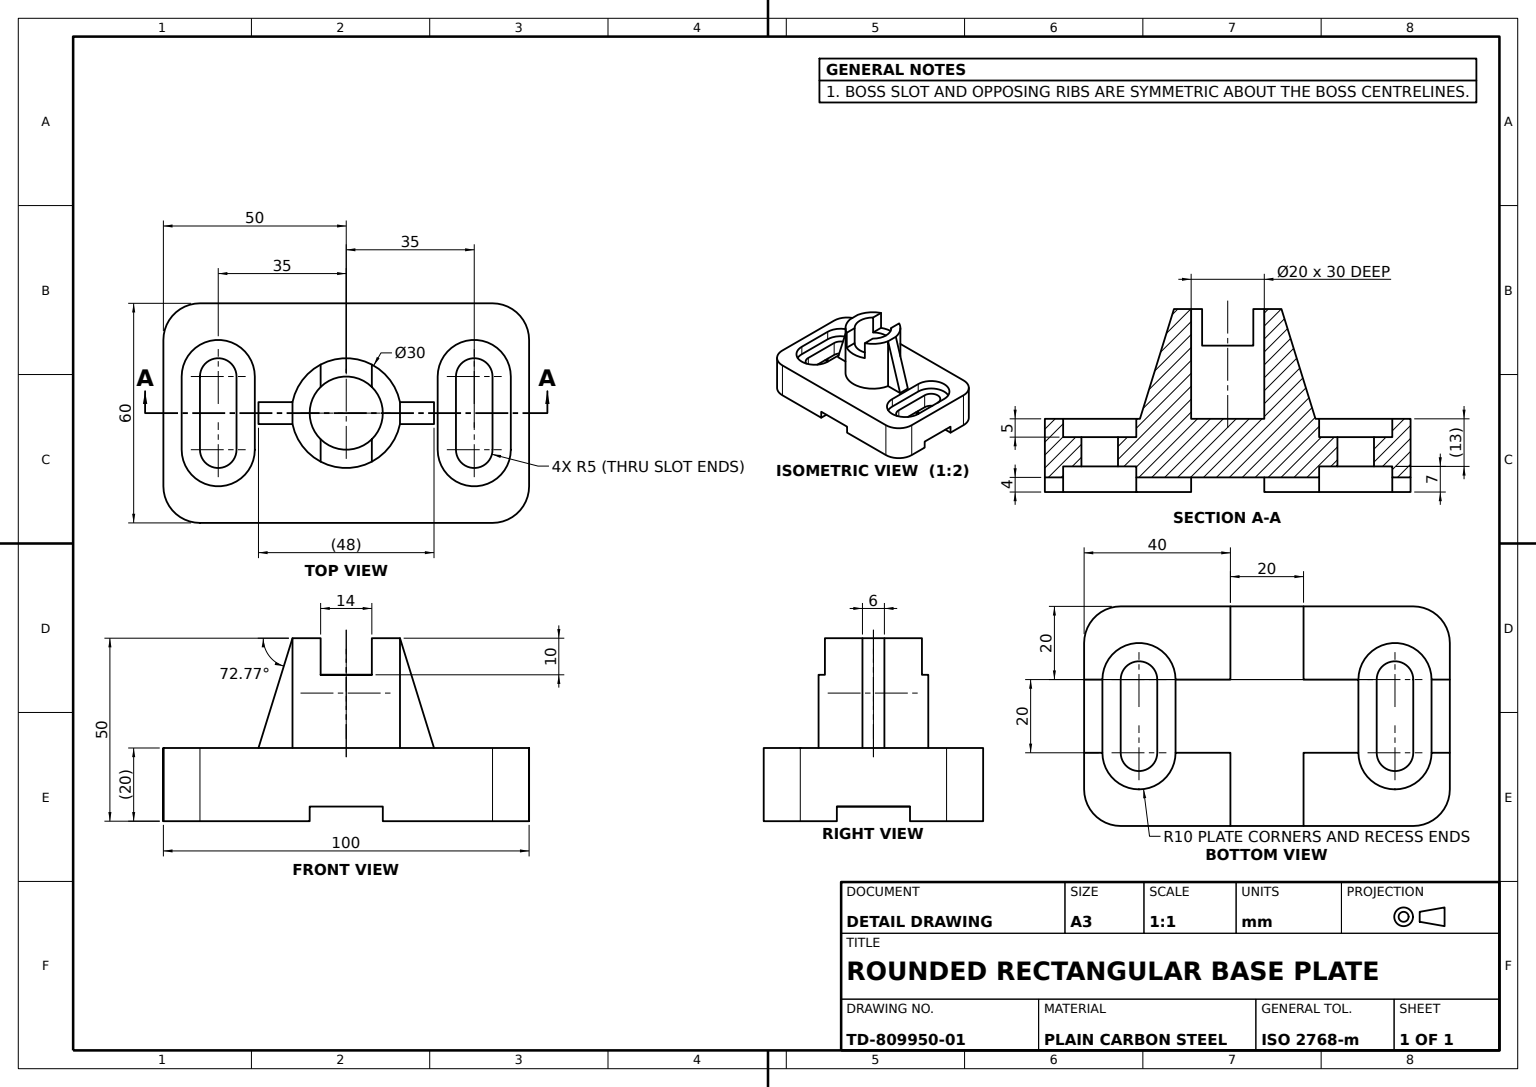
from build123d import *

# Parameters (mm, degrees)
BASE_PLATE_DEPTH         = 30
UNDERSIDE_NOTCHES_DEPTH  = 60
PIVOT_BOSS_SKETCH_R      = 15
PIVOT_BOSS_SKETCH_R_2    = 10
PIVOT_BOSS_30_DEPTH      = 30
SLOT_RECESS_A_DEPTH      = 13
SLOT_INNER_CUT_A_DEPTH   = 5
SLOT_START               = -7
SLOT_RECESS_B_DEPTH      = 7
SLOT_INNER_CUT_B_DEPTH   = 116.758369028
BOSS_SLOT_CUT_DEPTH      = 77.811457479
BOSS_SLOT_CUT_DEPTH_BACK = 77.811457479
SUPPORT_RIB_DEPTH        = 24
RIB_TRIM_CUT_DEPTH       = 77.811457479
RIB_TRIM_CUT_DEPTH_BACK  = 77.811457479
PIVOT_BORE_SKETCH_R      = 10
PIVOT_BORE_20_DEPTH      = 48


with BuildPart() as part:
    # Base Plate Profile Sketch → Base Plate (new, symmetric)
    with BuildSketch(Plane.XY):
        Polygon((-10, 4), (10, 4), (10, 0), (50, 0), (50, 20), (-50, 20), (-50, 0), (-10, 0), align=None)
    extrude(amount=BASE_PLATE_DEPTH, both=True)

    # Underside Notches Sketch → Underside Notches (cut)
    with BuildSketch(Plane(origin=(0, 20, 0), x_dir=(1, 0, 0), z_dir=(0, 1, 0))):
        with BuildLine():
            Line((40, 30), (50, 30))
            Line((50, 30), (50, 20))
            ThreePointArc((50, 20), (47.071067812, 27.071067812), (40, 30))
        make_face()
        with BuildLine():
            Line((-50, 30), (-50, 20))
            ThreePointArc((-50, 20), (-47.071067812, 27.071067812), (-40, 30))
            Line((-40, 30), (-50, 30))
        make_face()
        with BuildLine():
            Line((-50, -30), (-50, -20))
            ThreePointArc((-50, -20), (-47.071067812, -27.071067812), (-40, -30))
            Line((-40, -30), (-50, -30))
        make_face()
        with BuildLine():
            Line((50, -30), (50, -20))
            ThreePointArc((50, -20), (47.071067812, -27.071067812), (40, -30))
            Line((40, -30), (50, -30))
        make_face()
    extrude(amount=-UNDERSIDE_NOTCHES_DEPTH, mode=Mode.SUBTRACT)

    # Pivot Boss Sketch → Pivot Boss Ø30 (add)
    with BuildSketch(Plane(origin=(0, 20, 0), x_dir=(1, 0, 0), z_dir=(0, 1, 0))):
        Circle(PIVOT_BOSS_SKETCH_R)
        with Locations(Location((0, 0, 0), (0, 0, 180))):
            Circle(PIVOT_BOSS_SKETCH_R_2, mode=Mode.SUBTRACT)
    extrude(amount=PIVOT_BOSS_30_DEPTH)

    # Slot Recess A Sketch → Slot Recess A (cut)
    with BuildSketch(Plane(origin=(0, 20, 0), x_dir=(1, 0, 0), z_dir=(0, 1, 0))):
        with BuildLine():
            Line((30, -10), (30, 10))
            ThreePointArc((30, 10), (35, 15), (40, 10))
            Line((40, 10), (40, -10))
            ThreePointArc((40, -10), (35, -15), (30, -10))
        make_face()
        with BuildLine():
            Line((-30, -10), (-30, 10))
            ThreePointArc((-30, 10), (-35, 15), (-40, 10))
            Line((-40, 10), (-40, -10))
            ThreePointArc((-40, -10), (-35, -15), (-30, -10))
        make_face()
    extrude(amount=-SLOT_RECESS_A_DEPTH, mode=Mode.SUBTRACT)

    # Slot Inner Cut A Sketch → Slot Inner Cut A (cut)
    with BuildSketch(Plane(origin=(0, 20, 0), x_dir=(1, 0, 0), z_dir=(0, 1, 0))):
        with BuildLine():
            Line((25, -10), (25, 10))
            ThreePointArc((25, 10), (35, 20), (45, 10))
            Line((45, 10), (45, -10))
            ThreePointArc((45, -10), (35, -20), (25, -10))
        make_face()
        with BuildLine():
            Line((-25, -10), (-25, 10))
            ThreePointArc((-25, 10), (-35, 20), (-45, 10))
            Line((-45, 10), (-45, -10))
            ThreePointArc((-45, -10), (-35, -20), (-25, -10))
        make_face()
    extrude(amount=-SLOT_INNER_CUT_A_DEPTH, mode=Mode.SUBTRACT)

    # Slot Recess B Sketch → Slot Recess B (cut)
    with BuildSketch(Plane.XZ.offset(SLOT_START)):
        with BuildLine():
            Line((45, 10), (45, -10))
            ThreePointArc((45, -10), (35, -20), (25, -10))
            Line((25, -10), (25, 10))
            ThreePointArc((25, 10), (35, 20), (45, 10))
        make_face()
        with BuildLine():
            Line((-45, 10), (-45, -10))
            ThreePointArc((-45, -10), (-35, -20), (-25, -10))
            Line((-25, -10), (-25, 10))
            ThreePointArc((-25, 10), (-35, 20), (-45, 10))
        make_face()
    extrude(amount=SLOT_RECESS_B_DEPTH, mode=Mode.SUBTRACT)

    # Slot Inner Cut B Sketch → Slot Inner Cut B (cut, through all)
    with BuildSketch(Plane(origin=(50, 0, 0), x_dir=(0, 0, -1), z_dir=(1, 0, 0))):
        Polygon((0, 4), (10, 4), (10, 0), (-10, 0), (-10, 4), align=None)
    extrude(amount=-SLOT_INNER_CUT_B_DEPTH, mode=Mode.SUBTRACT)

    # Boss Slot Sketch → Boss Slot Cut (cut, two sides: drawn at the far end of the back side and taken through both)
    with BuildSketch(Plane.XY.offset(-BOSS_SLOT_CUT_DEPTH_BACK)):
        Polygon((0, 50), (7, 50), (7, 40), (-7, 40), (-7, 50), align=None)
    extrude(amount=BOSS_SLOT_CUT_DEPTH + BOSS_SLOT_CUT_DEPTH_BACK, mode=Mode.SUBTRACT)

    # Support Rib Sketch → Support Rib (add, symmetric)
    with BuildSketch(Plane(origin=(0, 0, 0), x_dir=(0, 0, -1), z_dir=(1, 0, 0))):
        Polygon((0, 50), (3, 50), (3, 20), (-3, 20), (-3, 50), align=None)
    extrude(amount=SUPPORT_RIB_DEPTH, both=True)

    # Rib Trim Sketch → Rib Trim Cut (cut, two sides: drawn at the far end of the back side and taken through both)
    with BuildSketch(Plane.XY.offset(-RIB_TRIM_CUT_DEPTH_BACK)):
        Polygon((24, 20), (14.696938457, 50), (24, 50), align=None)
        Polygon((-24, 50), (-24, 20), (-14.696938457, 50), align=None)
    extrude(amount=RIB_TRIM_CUT_DEPTH + RIB_TRIM_CUT_DEPTH_BACK, mode=Mode.SUBTRACT)

    # Pivot Bore Sketch → Pivot Bore Ø20 (cut)
    with BuildSketch(Plane(origin=(0, 20, 0), x_dir=(1, 0, 0), z_dir=(0, 1, 0))):
        with Locations(Location((0, 0, 0), (0, 0, 314.427004001))):
            Circle(PIVOT_BORE_SKETCH_R)
    extrude(amount=PIVOT_BORE_20_DEPTH, mode=Mode.SUBTRACT)


solid = part.part
